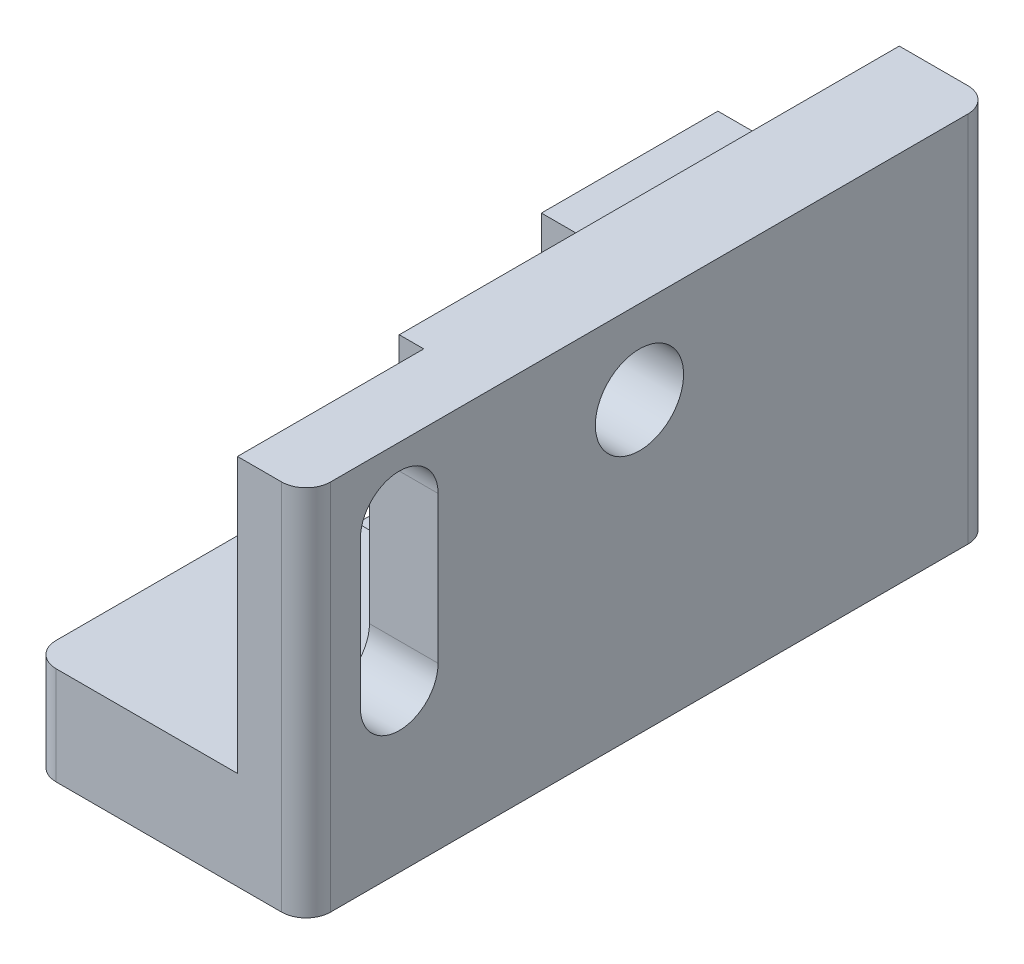
ISO-10303-21;
HEADER;
FILE_DESCRIPTION(('STEP AP214'),'2;1');
FILE_NAME('part.step','',(''),(''),'','','');
FILE_SCHEMA(('AUTOMOTIVE_DESIGN { 1 0 10303 214 1 1 1 1 }'));
ENDSEC;
DATA;
#1=APPLICATION_CONTEXT('core data for automotive mechanical design processes');
#2=APPLICATION_PROTOCOL_DEFINITION('international standard','automotive_design',2000,#1);
#3=PRODUCT_CONTEXT('',#1,'mechanical');
#4=PRODUCT('Part','Part','',(#3));
#5=PRODUCT_RELATED_PRODUCT_CATEGORY('part','',(#4));
#6=PRODUCT_DEFINITION_FORMATION('','',#4);
#7=PRODUCT_DEFINITION_CONTEXT('part definition',#1,'design');
#8=PRODUCT_DEFINITION('design','',#6,#7);
#9=PRODUCT_DEFINITION_SHAPE('','',#8);
#10=(LENGTH_UNIT() NAMED_UNIT(*) SI_UNIT(.MILLI.,.METRE.));
#11=(NAMED_UNIT(*) PLANE_ANGLE_UNIT() SI_UNIT($,.RADIAN.));
#12=(NAMED_UNIT(*) SI_UNIT($,.STERADIAN.) SOLID_ANGLE_UNIT());
#13=UNCERTAINTY_MEASURE_WITH_UNIT(LENGTH_MEASURE(1.E-05),#10,'distance_accuracy_value','');
#14=(GEOMETRIC_REPRESENTATION_CONTEXT(3) GLOBAL_UNCERTAINTY_ASSIGNED_CONTEXT((#13)) GLOBAL_UNIT_ASSIGNED_CONTEXT((#10,
#11,#12)) REPRESENTATION_CONTEXT('',''));
#15=CARTESIAN_POINT('',(0.,0.,0.));
#16=DIRECTION('',(0.,0.,1.));
#17=DIRECTION('',(1.,0.,0.));
#18=AXIS2_PLACEMENT_3D('',#15,#16,#17);
#19=CARTESIAN_POINT('',(-56.,20.,70.));
#20=DIRECTION('',(0.,-1.,0.));
#21=DIRECTION('',(0.,0.,-1.));
#22=AXIS2_PLACEMENT_3D('',#19,#20,#21);
#23=PLANE('',#22);
#24=DIRECTION('',(0.,0.,-1.));
#25=VECTOR('',#24,1.);
#26=CARTESIAN_POINT('',(-34.,20.,-16.4616556134456));
#27=LINE('',#26,#25);
#28=CARTESIAN_POINT('',(-34.,20.,13.5383443865544));
#29=VERTEX_POINT('',#28);
#30=CARTESIAN_POINT('',(-34.,20.,-16.4616556134456));
#31=VERTEX_POINT('',#30);
#32=EDGE_CURVE('E255',#29,#31,#27,.T.);
#33=ORIENTED_EDGE('',*,*,#32,.F.);
#34=DIRECTION('',(-1.,0.,0.));
#35=VECTOR('',#34,1.);
#36=CARTESIAN_POINT('',(-34.,20.,13.5383443865544));
#37=LINE('',#36,#35);
#38=CARTESIAN_POINT('',(-56.,20.,13.5383443865544));
#39=VERTEX_POINT('',#38);
#40=EDGE_CURVE('E269',#29,#39,#37,.T.);
#41=ORIENTED_EDGE('',*,*,#40,.T.);
#42=DIRECTION('',(0.,0.,-1.));
#43=VECTOR('',#42,1.);
#44=CARTESIAN_POINT('',(-56.,20.,70.));
#45=LINE('',#44,#43);
#46=CARTESIAN_POINT('',(-56.,20.,65.));
#47=VERTEX_POINT('',#46);
#48=EDGE_CURVE('E404',#47,#39,#45,.T.);
#49=ORIENTED_EDGE('',*,*,#48,.F.);
#50=CARTESIAN_POINT('',(-51.,20.,65.));
#51=DIRECTION('',(0.,-1.,0.));
#52=DIRECTION('',(0.,0.,1.));
#53=AXIS2_PLACEMENT_3D('',#50,#51,#52);
#54=CIRCLE('',#53,4.99999999999999);
#55=CARTESIAN_POINT('',(-51.,20.,70.));
#56=VERTEX_POINT('',#55);
#57=EDGE_CURVE('E352',#56,#47,#54,.T.);
#58=ORIENTED_EDGE('',*,*,#57,.F.);
#59=DIRECTION('',(-1.,0.,0.));
#60=VECTOR('',#59,1.);
#61=CARTESIAN_POINT('',(-56.,20.,70.));
#62=LINE('',#61,#60);
#63=CARTESIAN_POINT('',(-14.,20.,70.));
#64=VERTEX_POINT('',#63);
#65=EDGE_CURVE('E390',#64,#56,#62,.T.);
#66=ORIENTED_EDGE('',*,*,#65,.F.);
#67=DIRECTION('',(0.,0.,-1.));
#68=VECTOR('',#67,1.);
#69=CARTESIAN_POINT('',(-14.,20.,70.));
#70=LINE('',#69,#68);
#71=CARTESIAN_POINT('',(-14.,20.,32.));
#72=VERTEX_POINT('',#71);
#73=EDGE_CURVE('E410',#64,#72,#70,.T.);
#74=ORIENTED_EDGE('',*,*,#73,.T.);
#75=DIRECTION('',(1.,0.,0.));
#76=VECTOR('',#75,1.);
#77=CARTESIAN_POINT('',(-19.,20.,32.));
#78=LINE('',#77,#76);
#79=CARTESIAN_POINT('',(-19.,20.,32.));
#80=VERTEX_POINT('',#79);
#81=EDGE_CURVE('E351',#80,#72,#78,.T.);
#82=ORIENTED_EDGE('',*,*,#81,.F.);
#83=DIRECTION('',(0.,0.,1.));
#84=VECTOR('',#83,1.);
#85=CARTESIAN_POINT('',(-19.,20.,-70.));
#86=LINE('',#85,#84);
#87=CARTESIAN_POINT('',(-19.,20.,-34.));
#88=VERTEX_POINT('',#87);
#89=EDGE_CURVE('E339',#88,#80,#86,.T.);
#90=ORIENTED_EDGE('',*,*,#89,.F.);
#91=DIRECTION('',(-1.,0.,0.));
#92=VECTOR('',#91,1.);
#93=CARTESIAN_POINT('',(-19.,20.,-34.));
#94=LINE('',#93,#92);
#95=CARTESIAN_POINT('',(-56.,20.,-34.));
#96=VERTEX_POINT('',#95);
#97=EDGE_CURVE('E276',#88,#96,#94,.T.);
#98=ORIENTED_EDGE('',*,*,#97,.T.);
#99=CARTESIAN_POINT('',(-56.,20.,-16.4616556134456));
#100=VERTEX_POINT('',#99);
#101=EDGE_CURVE('E401',#100,#96,#45,.T.);
#102=ORIENTED_EDGE('',*,*,#101,.F.);
#103=DIRECTION('',(-1.,0.,0.));
#104=VECTOR('',#103,1.);
#105=CARTESIAN_POINT('',(-34.,20.,-16.4616556134456));
#106=LINE('',#105,#104);
#107=EDGE_CURVE('E65',#31,#100,#106,.T.);
#108=ORIENTED_EDGE('',*,*,#107,.F.);
#109=EDGE_LOOP('',(#33,#41,#49,#58,#66,#74,#82,#90,#98,#102,#108));
#110=FACE_BOUND('',#109,.T.);
#111=ADVANCED_FACE('F39',(#110),#23,.F.);
#112=CARTESIAN_POINT('',(-14.,20.,70.));
#113=DIRECTION('',(1.,0.,0.));
#114=DIRECTION('',(0.,0.,-1.));
#115=AXIS2_PLACEMENT_3D('',#112,#113,#114);
#116=PLANE('',#115);
#117=DIRECTION('',(0.,1.,0.));
#118=VECTOR('',#117,1.);
#119=CARTESIAN_POINT('',(-14.,33.,58.9234962612117));
#120=LINE('',#119,#118);
#121=CARTESIAN_POINT('',(-14.,33.,58.9234962612117));
#122=VERTEX_POINT('',#121);
#123=CARTESIAN_POINT('',(-14.,63.,58.9234962612117));
#124=VERTEX_POINT('',#123);
#125=EDGE_CURVE('E318',#122,#124,#120,.T.);
#126=ORIENTED_EDGE('',*,*,#125,.F.);
#127=CARTESIAN_POINT('',(-14.,33.,51.));
#128=DIRECTION('',(-1.,0.,0.));
#129=DIRECTION('',(0.,0.,1.));
#130=AXIS2_PLACEMENT_3D('',#127,#128,#129);
#131=CIRCLE('',#130,7.92349626121171);
#132=CARTESIAN_POINT('',(-14.,33.,43.0765037387883));
#133=VERTEX_POINT('',#132);
#134=EDGE_CURVE('E305',#133,#122,#131,.T.);
#135=ORIENTED_EDGE('',*,*,#134,.F.);
#136=DIRECTION('',(0.,-1.,0.));
#137=VECTOR('',#136,1.);
#138=CARTESIAN_POINT('',(-14.,33.,43.0765037387883));
#139=LINE('',#138,#137);
#140=CARTESIAN_POINT('',(-14.,63.,43.0765037387883));
#141=VERTEX_POINT('',#140);
#142=EDGE_CURVE('E307',#141,#133,#139,.T.);
#143=ORIENTED_EDGE('',*,*,#142,.F.);
#144=CARTESIAN_POINT('',(-14.,63.,51.));
#145=DIRECTION('',(-1.,0.,0.));
#146=DIRECTION('',(0.,0.,1.));
#147=AXIS2_PLACEMENT_3D('',#144,#145,#146);
#148=CIRCLE('',#147,7.92349626121171);
#149=EDGE_CURVE('E324',#124,#141,#148,.T.);
#150=ORIENTED_EDGE('',*,*,#149,.F.);
#151=EDGE_LOOP('',(#126,#135,#143,#150));
#152=FACE_BOUND('',#151,.T.);
#153=DIRECTION('',(0.,1.,0.));
#154=VECTOR('',#153,1.);
#155=CARTESIAN_POINT('',(-14.,76.,32.));
#156=LINE('',#155,#154);
#157=CARTESIAN_POINT('',(-14.,76.,32.));
#158=VERTEX_POINT('',#157);
#159=EDGE_CURVE('E326',#72,#158,#156,.T.);
#160=ORIENTED_EDGE('',*,*,#159,.F.);
#161=ORIENTED_EDGE('',*,*,#73,.F.);
#162=DIRECTION('',(0.,-1.,0.));
#163=VECTOR('',#162,1.);
#164=CARTESIAN_POINT('',(-14.,20.,70.));
#165=LINE('',#164,#163);
#166=CARTESIAN_POINT('',(-14.,76.,70.));
#167=VERTEX_POINT('',#166);
#168=EDGE_CURVE('E381',#167,#64,#165,.T.);
#169=ORIENTED_EDGE('',*,*,#168,.F.);
#170=DIRECTION('',(0.,0.,-1.));
#171=VECTOR('',#170,1.);
#172=CARTESIAN_POINT('',(-14.,76.,70.));
#173=LINE('',#172,#171);
#174=EDGE_CURVE('E408',#167,#158,#173,.T.);
#175=ORIENTED_EDGE('',*,*,#174,.T.);
#176=EDGE_LOOP('',(#160,#161,#169,#175));
#177=FACE_BOUND('',#176,.T.);
#178=ADVANCED_FACE('F450',(#152,#177),#116,.F.);
#179=CARTESIAN_POINT('',(-56.,0.,70.));
#180=DIRECTION('',(1.,0.,0.));
#181=DIRECTION('',(0.,0.,-1.));
#182=AXIS2_PLACEMENT_3D('',#179,#180,#181);
#183=PLANE('',#182);
#184=ORIENTED_EDGE('',*,*,#48,.T.);
#185=DIRECTION('',(0.,1.,0.));
#186=VECTOR('',#185,1.);
#187=CARTESIAN_POINT('',(-56.,9.99999999999999,13.5383443865544));
#188=LINE('',#187,#186);
#189=CARTESIAN_POINT('',(-56.,9.99999999999999,13.5383443865544));
#190=VERTEX_POINT('',#189);
#191=EDGE_CURVE('E257',#190,#39,#188,.T.);
#192=ORIENTED_EDGE('',*,*,#191,.F.);
#193=DIRECTION('',(0.,0.,1.));
#194=VECTOR('',#193,1.);
#195=CARTESIAN_POINT('',(-56.,9.99999999999999,-16.4616556134456));
#196=LINE('',#195,#194);
#197=CARTESIAN_POINT('',(-56.,9.99999999999999,-16.4616556134456));
#198=VERTEX_POINT('',#197);
#199=EDGE_CURVE('E266',#198,#190,#196,.T.);
#200=ORIENTED_EDGE('',*,*,#199,.F.);
#201=DIRECTION('',(0.,-1.,0.));
#202=VECTOR('',#201,1.);
#203=CARTESIAN_POINT('',(-56.,20.,-16.4616556134456));
#204=LINE('',#203,#202);
#205=EDGE_CURVE('E252',#100,#198,#204,.T.);
#206=ORIENTED_EDGE('',*,*,#205,.F.);
#207=ORIENTED_EDGE('',*,*,#101,.T.);
#208=DIRECTION('',(0.,1.,0.));
#209=VECTOR('',#208,1.);
#210=CARTESIAN_POINT('',(-56.,20.,-34.));
#211=LINE('',#210,#209);
#212=CARTESIAN_POINT('',(-56.,46.,-34.));
#213=VERTEX_POINT('',#212);
#214=EDGE_CURVE('E285',#96,#213,#211,.T.);
#215=ORIENTED_EDGE('',*,*,#214,.T.);
#216=DIRECTION('',(0.,0.,-1.));
#217=VECTOR('',#216,1.);
#218=CARTESIAN_POINT('',(-56.,46.,-34.));
#219=LINE('',#218,#217);
#220=CARTESIAN_POINT('',(-56.,46.,-70.));
#221=VERTEX_POINT('',#220);
#222=EDGE_CURVE('E289',#213,#221,#219,.T.);
#223=ORIENTED_EDGE('',*,*,#222,.T.);
#224=DIRECTION('',(0.,-1.,0.));
#225=VECTOR('',#224,1.);
#226=CARTESIAN_POINT('',(-56.,0.,-70.));
#227=LINE('',#226,#225);
#228=CARTESIAN_POINT('',(-56.,0.,-70.));
#229=VERTEX_POINT('',#228);
#230=EDGE_CURVE('E394',#221,#229,#227,.T.);
#231=ORIENTED_EDGE('',*,*,#230,.T.);
#232=DIRECTION('',(0.,0.,-1.));
#233=VECTOR('',#232,1.);
#234=CARTESIAN_POINT('',(-56.,0.,70.));
#235=LINE('',#234,#233);
#236=CARTESIAN_POINT('',(-56.,0.,65.));
#237=VERTEX_POINT('',#236);
#238=EDGE_CURVE('E402',#237,#229,#235,.T.);
#239=ORIENTED_EDGE('',*,*,#238,.F.);
#240=DIRECTION('',(0.,1.,0.));
#241=VECTOR('',#240,1.);
#242=CARTESIAN_POINT('',(-56.,-120.,65.));
#243=LINE('',#242,#241);
#244=EDGE_CURVE('E357',#237,#47,#243,.T.);
#245=ORIENTED_EDGE('',*,*,#244,.T.);
#246=EDGE_LOOP('',(#184,#192,#200,#206,#207,#215,#223,#231,#239,#245));
#247=FACE_BOUND('',#246,.T.);
#248=ADVANCED_FACE('F460',(#247),#183,.F.);
#249=CARTESIAN_POINT('',(0.,0.,70.));
#250=DIRECTION('',(0.,1.,0.));
#251=DIRECTION('',(-1.,0.,0.));
#252=AXIS2_PLACEMENT_3D('',#249,#250,#251);
#253=PLANE('',#252);
#254=CARTESIAN_POINT('',(-44.724100920092,0.,-1.46165561344556));
#255=DIRECTION('',(0.,1.,0.));
#256=DIRECTION('',(-1.,0.,0.));
#257=AXIS2_PLACEMENT_3D('',#254,#255,#256);
#258=CIRCLE('',#257,6.);
#259=CARTESIAN_POINT('',(-50.724100920092,0.,-1.46165561344556));
#260=VERTEX_POINT('',#259);
#261=EDGE_CURVE('E247',#260,#260,#258,.T.);
#262=ORIENTED_EDGE('',*,*,#261,.T.);
#263=EDGE_LOOP('',(#262));
#264=FACE_BOUND('',#263,.T.);
#265=DIRECTION('',(1.,0.,0.));
#266=VECTOR('',#265,1.);
#267=CARTESIAN_POINT('',(0.,0.,70.));
#268=LINE('',#267,#266);
#269=CARTESIAN_POINT('',(-51.,0.,70.));
#270=VERTEX_POINT('',#269);
#271=CARTESIAN_POINT('',(-5.,0.,70.));
#272=VERTEX_POINT('',#271);
#273=EDGE_CURVE('E388',#270,#272,#268,.T.);
#274=ORIENTED_EDGE('',*,*,#273,.F.);
#275=CARTESIAN_POINT('',(-51.,0.,65.));
#276=DIRECTION('',(0.,1.,0.));
#277=DIRECTION('',(-1.,0.,0.));
#278=AXIS2_PLACEMENT_3D('',#275,#276,#277);
#279=CIRCLE('',#278,4.99999999999999);
#280=EDGE_CURVE('E11',#270,#237,#279,.F.);
#281=ORIENTED_EDGE('',*,*,#280,.T.);
#282=ORIENTED_EDGE('',*,*,#238,.T.);
#283=DIRECTION('',(1.,0.,0.));
#284=VECTOR('',#283,1.);
#285=CARTESIAN_POINT('',(0.,0.,-70.));
#286=LINE('',#285,#284);
#287=CARTESIAN_POINT('',(-5.,0.,-70.));
#288=VERTEX_POINT('',#287);
#289=EDGE_CURVE('E383',#229,#288,#286,.T.);
#290=ORIENTED_EDGE('',*,*,#289,.T.);
#291=CARTESIAN_POINT('',(-5.,0.,-65.));
#292=DIRECTION('',(0.,-1.,0.));
#293=DIRECTION('',(0.,0.,1.));
#294=AXIS2_PLACEMENT_3D('',#291,#292,#293);
#295=CIRCLE('',#294,5.);
#296=CARTESIAN_POINT('',(0.,0.,-65.));
#297=VERTEX_POINT('',#296);
#298=EDGE_CURVE('E365',#288,#297,#295,.T.);
#299=ORIENTED_EDGE('',*,*,#298,.T.);
#300=DIRECTION('',(0.,0.,-1.));
#301=VECTOR('',#300,1.);
#302=CARTESIAN_POINT('',(0.,0.,70.));
#303=LINE('',#302,#301);
#304=CARTESIAN_POINT('',(0.,0.,65.));
#305=VERTEX_POINT('',#304);
#306=EDGE_CURVE('E395',#305,#297,#303,.T.);
#307=ORIENTED_EDGE('',*,*,#306,.F.);
#308=CARTESIAN_POINT('',(-5.,0.,65.));
#309=DIRECTION('',(0.,-1.,0.));
#310=DIRECTION('',(0.,0.,-1.));
#311=AXIS2_PLACEMENT_3D('',#308,#309,#310);
#312=CIRCLE('',#311,5.);
#313=EDGE_CURVE('E372',#305,#272,#312,.T.);
#314=ORIENTED_EDGE('',*,*,#313,.T.);
#315=EDGE_LOOP('',(#274,#281,#282,#290,#299,#307,#314));
#316=FACE_BOUND('',#315,.T.);
#317=ADVANCED_FACE('F430',(#264,#316),#253,.F.);
#318=CARTESIAN_POINT('',(0.,76.,70.));
#319=DIRECTION('',(-1.,0.,0.));
#320=DIRECTION('',(0.,0.,1.));
#321=AXIS2_PLACEMENT_3D('',#318,#319,#320);
#322=PLANE('',#321);
#323=CARTESIAN_POINT('',(0.,59.,2.00000000000001));
#324=DIRECTION('',(-1.,0.,0.));
#325=DIRECTION('',(0.,0.,1.));
#326=AXIS2_PLACEMENT_3D('',#323,#324,#325);
#327=CIRCLE('',#326,9.);
#328=CARTESIAN_POINT('',(0.,59.,11.));
#329=VERTEX_POINT('',#328);
#330=EDGE_CURVE('E299',#329,#329,#327,.T.);
#331=ORIENTED_EDGE('',*,*,#330,.T.);
#332=EDGE_LOOP('',(#331));
#333=FACE_BOUND('',#332,.T.);
#334=DIRECTION('',(0.,-1.,0.));
#335=VECTOR('',#334,1.);
#336=CARTESIAN_POINT('',(0.,33.,43.0765037387883));
#337=LINE('',#336,#335);
#338=CARTESIAN_POINT('',(0.,63.,43.0765037387883));
#339=VERTEX_POINT('',#338);
#340=CARTESIAN_POINT('',(0.,33.,43.0765037387883));
#341=VERTEX_POINT('',#340);
#342=EDGE_CURVE('E314',#339,#341,#337,.T.);
#343=ORIENTED_EDGE('',*,*,#342,.T.);
#344=CARTESIAN_POINT('',(0.,33.,51.));
#345=DIRECTION('',(-1.,0.,0.));
#346=DIRECTION('',(0.,0.,1.));
#347=AXIS2_PLACEMENT_3D('',#344,#345,#346);
#348=CIRCLE('',#347,7.92349626121171);
#349=CARTESIAN_POINT('',(0.,33.,58.9234962612117));
#350=VERTEX_POINT('',#349);
#351=EDGE_CURVE('E304',#341,#350,#348,.T.);
#352=ORIENTED_EDGE('',*,*,#351,.T.);
#353=DIRECTION('',(0.,1.,0.));
#354=VECTOR('',#353,1.);
#355=CARTESIAN_POINT('',(0.,33.,58.9234962612117));
#356=LINE('',#355,#354);
#357=CARTESIAN_POINT('',(0.,63.,58.9234962612117));
#358=VERTEX_POINT('',#357);
#359=EDGE_CURVE('E308',#350,#358,#356,.T.);
#360=ORIENTED_EDGE('',*,*,#359,.T.);
#361=CARTESIAN_POINT('',(0.,63.,51.));
#362=DIRECTION('',(-1.,0.,0.));
#363=DIRECTION('',(0.,0.,1.));
#364=AXIS2_PLACEMENT_3D('',#361,#362,#363);
#365=CIRCLE('',#364,7.92349626121171);
#366=EDGE_CURVE('E315',#358,#339,#365,.T.);
#367=ORIENTED_EDGE('',*,*,#366,.T.);
#368=EDGE_LOOP('',(#343,#352,#360,#367));
#369=FACE_BOUND('',#368,.T.);
#370=DIRECTION('',(0.,1.,0.));
#371=VECTOR('',#370,1.);
#372=CARTESIAN_POINT('',(0.,0.,-65.));
#373=LINE('',#372,#371);
#374=CARTESIAN_POINT('',(0.,76.,-65.));
#375=VERTEX_POINT('',#374);
#376=EDGE_CURVE('E367',#297,#375,#373,.T.);
#377=ORIENTED_EDGE('',*,*,#376,.T.);
#378=DIRECTION('',(0.,0.,-1.));
#379=VECTOR('',#378,1.);
#380=CARTESIAN_POINT('',(0.,76.,70.));
#381=LINE('',#380,#379);
#382=CARTESIAN_POINT('',(0.,76.,65.));
#383=VERTEX_POINT('',#382);
#384=EDGE_CURVE('E50',#383,#375,#381,.T.);
#385=ORIENTED_EDGE('',*,*,#384,.F.);
#386=DIRECTION('',(0.,1.,0.));
#387=VECTOR('',#386,1.);
#388=CARTESIAN_POINT('',(0.,0.,65.));
#389=LINE('',#388,#387);
#390=EDGE_CURVE('E380',#305,#383,#389,.T.);
#391=ORIENTED_EDGE('',*,*,#390,.F.);
#392=ORIENTED_EDGE('',*,*,#306,.T.);
#393=EDGE_LOOP('',(#377,#385,#391,#392));
#394=FACE_BOUND('',#393,.T.);
#395=ADVANCED_FACE('F41',(#333,#369,#394),#322,.F.);
#396=CARTESIAN_POINT('',(0.,0.,70.));
#397=DIRECTION('',(0.,0.,-1.));
#398=DIRECTION('',(-1.,0.,0.));
#399=AXIS2_PLACEMENT_3D('',#396,#397,#398);
#400=PLANE('',#399);
#401=ORIENTED_EDGE('',*,*,#65,.T.);
#402=DIRECTION('',(0.,1.,0.));
#403=VECTOR('',#402,1.);
#404=CARTESIAN_POINT('',(-51.,-120.,70.));
#405=LINE('',#404,#403);
#406=EDGE_CURVE('E358',#270,#56,#405,.T.);
#407=ORIENTED_EDGE('',*,*,#406,.F.);
#408=ORIENTED_EDGE('',*,*,#273,.T.);
#409=DIRECTION('',(0.,1.,0.));
#410=VECTOR('',#409,1.);
#411=CARTESIAN_POINT('',(-5.,0.,70.));
#412=LINE('',#411,#410);
#413=CARTESIAN_POINT('',(-5.,76.,70.));
#414=VERTEX_POINT('',#413);
#415=EDGE_CURVE('E368',#272,#414,#412,.T.);
#416=ORIENTED_EDGE('',*,*,#415,.T.);
#417=DIRECTION('',(-1.,0.,0.));
#418=VECTOR('',#417,1.);
#419=CARTESIAN_POINT('',(-14.,76.,70.));
#420=LINE('',#419,#418);
#421=EDGE_CURVE('E385',#414,#167,#420,.T.);
#422=ORIENTED_EDGE('',*,*,#421,.T.);
#423=ORIENTED_EDGE('',*,*,#168,.T.);
#424=EDGE_LOOP('',(#401,#407,#408,#416,#422,#423));
#425=FACE_BOUND('',#424,.T.);
#426=ADVANCED_FACE('F448',(#425),#400,.F.);
#427=CARTESIAN_POINT('',(0.,0.,-70.));
#428=DIRECTION('',(0.,0.,-1.));
#429=DIRECTION('',(-1.,0.,0.));
#430=AXIS2_PLACEMENT_3D('',#427,#428,#429);
#431=PLANE('',#430);
#432=ORIENTED_EDGE('',*,*,#230,.F.);
#433=DIRECTION('',(1.,0.,0.));
#434=VECTOR('',#433,1.);
#435=CARTESIAN_POINT('',(-56.,46.,-70.));
#436=LINE('',#435,#434);
#437=CARTESIAN_POINT('',(-19.,46.,-70.));
#438=VERTEX_POINT('',#437);
#439=EDGE_CURVE('E271',#221,#438,#436,.T.);
#440=ORIENTED_EDGE('',*,*,#439,.T.);
#441=DIRECTION('',(0.,-1.,0.));
#442=VECTOR('',#441,1.);
#443=CARTESIAN_POINT('',(-19.,76.,-70.));
#444=LINE('',#443,#442);
#445=CARTESIAN_POINT('',(-19.,76.,-70.));
#446=VERTEX_POINT('',#445);
#447=EDGE_CURVE('E340',#446,#438,#444,.T.);
#448=ORIENTED_EDGE('',*,*,#447,.F.);
#449=DIRECTION('',(-1.,0.,0.));
#450=VECTOR('',#449,1.);
#451=CARTESIAN_POINT('',(-14.,76.,-70.));
#452=LINE('',#451,#450);
#453=CARTESIAN_POINT('',(-5.,76.,-70.));
#454=VERTEX_POINT('',#453);
#455=EDGE_CURVE('E375',#454,#446,#452,.T.);
#456=ORIENTED_EDGE('',*,*,#455,.F.);
#457=DIRECTION('',(0.,1.,0.));
#458=VECTOR('',#457,1.);
#459=CARTESIAN_POINT('',(-5.,0.,-70.));
#460=LINE('',#459,#458);
#461=EDGE_CURVE('E362',#288,#454,#460,.T.);
#462=ORIENTED_EDGE('',*,*,#461,.F.);
#463=ORIENTED_EDGE('',*,*,#289,.F.);
#464=EDGE_LOOP('',(#432,#440,#448,#456,#462,#463));
#465=FACE_BOUND('',#464,.T.);
#466=ADVANCED_FACE('F431',(#465),#431,.T.);
#467=CARTESIAN_POINT('',(-14.,76.,70.));
#468=DIRECTION('',(0.,-1.,0.));
#469=DIRECTION('',(0.,0.,-1.));
#470=AXIS2_PLACEMENT_3D('',#467,#468,#469);
#471=PLANE('',#470);
#472=ORIENTED_EDGE('',*,*,#384,.T.);
#473=CARTESIAN_POINT('',(-5.,76.,-65.));
#474=DIRECTION('',(0.,-1.,0.));
#475=DIRECTION('',(0.,0.,1.));
#476=AXIS2_PLACEMENT_3D('',#473,#474,#475);
#477=CIRCLE('',#476,5.);
#478=EDGE_CURVE('E366',#454,#375,#477,.T.);
#479=ORIENTED_EDGE('',*,*,#478,.F.);
#480=ORIENTED_EDGE('',*,*,#455,.T.);
#481=DIRECTION('',(0.,0.,-1.));
#482=VECTOR('',#481,1.);
#483=CARTESIAN_POINT('',(-19.,76.,32.));
#484=LINE('',#483,#482);
#485=CARTESIAN_POINT('',(-19.,76.,32.));
#486=VERTEX_POINT('',#485);
#487=EDGE_CURVE('E344',#486,#446,#484,.T.);
#488=ORIENTED_EDGE('',*,*,#487,.F.);
#489=DIRECTION('',(1.,0.,0.));
#490=VECTOR('',#489,1.);
#491=CARTESIAN_POINT('',(-19.,76.,32.));
#492=LINE('',#491,#490);
#493=EDGE_CURVE('E347',#486,#158,#492,.T.);
#494=ORIENTED_EDGE('',*,*,#493,.T.);
#495=ORIENTED_EDGE('',*,*,#174,.F.);
#496=ORIENTED_EDGE('',*,*,#421,.F.);
#497=CARTESIAN_POINT('',(-5.,76.,65.));
#498=DIRECTION('',(0.,-1.,0.));
#499=DIRECTION('',(0.,0.,-1.));
#500=AXIS2_PLACEMENT_3D('',#497,#498,#499);
#501=CIRCLE('',#500,5.);
#502=EDGE_CURVE('E359',#383,#414,#501,.T.);
#503=ORIENTED_EDGE('',*,*,#502,.F.);
#504=EDGE_LOOP('',(#472,#479,#480,#488,#494,#495,#496,#503));
#505=FACE_BOUND('',#504,.T.);
#506=ADVANCED_FACE('F416',(#505),#471,.F.);
#507=CARTESIAN_POINT('',(-5.,0.,-65.));
#508=DIRECTION('',(0.,1.,0.));
#509=DIRECTION('',(0.,0.,1.));
#510=AXIS2_PLACEMENT_3D('',#507,#508,#509);
#511=CYLINDRICAL_SURFACE('',#510,5.);
#512=ORIENTED_EDGE('',*,*,#478,.T.);
#513=ORIENTED_EDGE('',*,*,#376,.F.);
#514=ORIENTED_EDGE('',*,*,#298,.F.);
#515=ORIENTED_EDGE('',*,*,#461,.T.);
#516=EDGE_LOOP('',(#512,#513,#514,#515));
#517=FACE_BOUND('',#516,.T.);
#518=ADVANCED_FACE('F421',(#517),#511,.T.);
#519=CARTESIAN_POINT('',(-5.,0.,65.));
#520=DIRECTION('',(0.,1.,0.));
#521=DIRECTION('',(0.,0.,1.));
#522=AXIS2_PLACEMENT_3D('',#519,#520,#521);
#523=CYLINDRICAL_SURFACE('',#522,5.);
#524=ORIENTED_EDGE('',*,*,#502,.T.);
#525=ORIENTED_EDGE('',*,*,#415,.F.);
#526=ORIENTED_EDGE('',*,*,#313,.F.);
#527=ORIENTED_EDGE('',*,*,#390,.T.);
#528=EDGE_LOOP('',(#524,#525,#526,#527));
#529=FACE_BOUND('',#528,.T.);
#530=ADVANCED_FACE('F451',(#529),#523,.T.);
#531=CARTESIAN_POINT('',(-51.,-120.,65.));
#532=DIRECTION('',(0.,1.,0.));
#533=DIRECTION('',(0.,0.,1.));
#534=AXIS2_PLACEMENT_3D('',#531,#532,#533);
#535=CYLINDRICAL_SURFACE('',#534,4.99999999999999);
#536=ORIENTED_EDGE('',*,*,#406,.T.);
#537=ORIENTED_EDGE('',*,*,#57,.T.);
#538=ORIENTED_EDGE('',*,*,#244,.F.);
#539=ORIENTED_EDGE('',*,*,#280,.F.);
#540=EDGE_LOOP('',(#536,#537,#538,#539));
#541=FACE_BOUND('',#540,.T.);
#542=ADVANCED_FACE('F546',(#541),#535,.T.);
#543=CARTESIAN_POINT('',(-19.,76.,32.));
#544=DIRECTION('',(0.,0.,-1.));
#545=DIRECTION('',(-1.,0.,0.));
#546=AXIS2_PLACEMENT_3D('',#543,#544,#545);
#547=PLANE('',#546);
#548=ORIENTED_EDGE('',*,*,#159,.T.);
#549=ORIENTED_EDGE('',*,*,#493,.F.);
#550=DIRECTION('',(0.,1.,0.));
#551=VECTOR('',#550,1.);
#552=CARTESIAN_POINT('',(-19.,76.,32.));
#553=LINE('',#552,#551);
#554=EDGE_CURVE('E342',#80,#486,#553,.T.);
#555=ORIENTED_EDGE('',*,*,#554,.F.);
#556=ORIENTED_EDGE('',*,*,#81,.T.);
#557=EDGE_LOOP('',(#548,#549,#555,#556));
#558=FACE_BOUND('',#557,.T.);
#559=ADVANCED_FACE('F445',(#558),#547,.F.);
#560=CARTESIAN_POINT('',(-19.,0.,0.));
#561=DIRECTION('',(-1.,0.,0.));
#562=DIRECTION('',(0.,0.,1.));
#563=AXIS2_PLACEMENT_3D('',#560,#561,#562);
#564=PLANE('',#563);
#565=DIRECTION('',(0.,0.,-1.));
#566=VECTOR('',#565,1.);
#567=CARTESIAN_POINT('',(-19.,46.,-34.));
#568=LINE('',#567,#566);
#569=CARTESIAN_POINT('',(-19.,46.,-34.));
#570=VERTEX_POINT('',#569);
#571=EDGE_CURVE('E291',#570,#438,#568,.T.);
#572=ORIENTED_EDGE('',*,*,#571,.F.);
#573=DIRECTION('',(0.,-1.,0.));
#574=VECTOR('',#573,1.);
#575=CARTESIAN_POINT('',(-19.,46.,-34.));
#576=LINE('',#575,#574);
#577=EDGE_CURVE('E288',#570,#88,#576,.T.);
#578=ORIENTED_EDGE('',*,*,#577,.T.);
#579=ORIENTED_EDGE('',*,*,#89,.T.);
#580=ORIENTED_EDGE('',*,*,#554,.T.);
#581=ORIENTED_EDGE('',*,*,#487,.T.);
#582=ORIENTED_EDGE('',*,*,#447,.T.);
#583=EDGE_LOOP('',(#572,#578,#579,#580,#581,#582));
#584=FACE_BOUND('',#583,.T.);
#585=CARTESIAN_POINT('',(-19.,59.,2.00000000000001));
#586=DIRECTION('',(-1.,0.,0.));
#587=DIRECTION('',(0.,0.,1.));
#588=AXIS2_PLACEMENT_3D('',#585,#586,#587);
#589=CIRCLE('',#588,9.);
#590=CARTESIAN_POINT('',(-19.,59.,11.));
#591=VERTEX_POINT('',#590);
#592=EDGE_CURVE('E298',#591,#591,#589,.T.);
#593=ORIENTED_EDGE('',*,*,#592,.F.);
#594=EDGE_LOOP('',(#593));
#595=FACE_BOUND('',#594,.T.);
#596=ADVANCED_FACE('F434',(#584,#595),#564,.T.);
#597=CARTESIAN_POINT('',(0.,33.,51.));
#598=DIRECTION('',(-1.,0.,0.));
#599=DIRECTION('',(0.,0.,1.));
#600=AXIS2_PLACEMENT_3D('',#597,#598,#599);
#601=CYLINDRICAL_SURFACE('',#600,7.92349626121171);
#602=ORIENTED_EDGE('',*,*,#134,.T.);
#603=DIRECTION('',(-1.,0.,0.));
#604=VECTOR('',#603,1.);
#605=CARTESIAN_POINT('',(0.,33.,58.9234962612117));
#606=LINE('',#605,#604);
#607=EDGE_CURVE('E319',#350,#122,#606,.T.);
#608=ORIENTED_EDGE('',*,*,#607,.F.);
#609=ORIENTED_EDGE('',*,*,#351,.F.);
#610=DIRECTION('',(-1.,0.,0.));
#611=VECTOR('',#610,1.);
#612=CARTESIAN_POINT('',(0.,33.,43.0765037387883));
#613=LINE('',#612,#611);
#614=EDGE_CURVE('E328',#341,#133,#613,.T.);
#615=ORIENTED_EDGE('',*,*,#614,.T.);
#616=EDGE_LOOP('',(#602,#608,#609,#615));
#617=FACE_BOUND('',#616,.T.);
#618=ADVANCED_FACE('F555',(#617),#601,.F.);
#619=CARTESIAN_POINT('',(0.,33.,43.0765037387883));
#620=DIRECTION('',(0.,0.,-1.));
#621=DIRECTION('',(0.,1.,0.));
#622=AXIS2_PLACEMENT_3D('',#619,#620,#621);
#623=PLANE('',#622);
#624=ORIENTED_EDGE('',*,*,#142,.T.);
#625=ORIENTED_EDGE('',*,*,#614,.F.);
#626=ORIENTED_EDGE('',*,*,#342,.F.);
#627=DIRECTION('',(-1.,0.,0.));
#628=VECTOR('',#627,1.);
#629=CARTESIAN_POINT('',(0.,63.,43.0765037387883));
#630=LINE('',#629,#628);
#631=EDGE_CURVE('E331',#339,#141,#630,.T.);
#632=ORIENTED_EDGE('',*,*,#631,.T.);
#633=EDGE_LOOP('',(#624,#625,#626,#632));
#634=FACE_BOUND('',#633,.T.);
#635=ADVANCED_FACE('F560',(#634),#623,.F.);
#636=CARTESIAN_POINT('',(0.,63.,51.));
#637=DIRECTION('',(-1.,0.,0.));
#638=DIRECTION('',(0.,0.,1.));
#639=AXIS2_PLACEMENT_3D('',#636,#637,#638);
#640=CYLINDRICAL_SURFACE('',#639,7.92349626121171);
#641=ORIENTED_EDGE('',*,*,#149,.T.);
#642=ORIENTED_EDGE('',*,*,#631,.F.);
#643=ORIENTED_EDGE('',*,*,#366,.F.);
#644=DIRECTION('',(-1.,0.,0.));
#645=VECTOR('',#644,1.);
#646=CARTESIAN_POINT('',(0.,63.,58.9234962612117));
#647=LINE('',#646,#645);
#648=EDGE_CURVE('E333',#358,#124,#647,.T.);
#649=ORIENTED_EDGE('',*,*,#648,.T.);
#650=EDGE_LOOP('',(#641,#642,#643,#649));
#651=FACE_BOUND('',#650,.T.);
#652=ADVANCED_FACE('F565',(#651),#640,.F.);
#653=CARTESIAN_POINT('',(0.,33.,58.9234962612117));
#654=DIRECTION('',(0.,0.,1.));
#655=DIRECTION('',(0.,-1.,0.));
#656=AXIS2_PLACEMENT_3D('',#653,#654,#655);
#657=PLANE('',#656);
#658=ORIENTED_EDGE('',*,*,#125,.T.);
#659=ORIENTED_EDGE('',*,*,#648,.F.);
#660=ORIENTED_EDGE('',*,*,#359,.F.);
#661=ORIENTED_EDGE('',*,*,#607,.T.);
#662=EDGE_LOOP('',(#658,#659,#660,#661));
#663=FACE_BOUND('',#662,.T.);
#664=ADVANCED_FACE('F559',(#663),#657,.F.);
#665=CARTESIAN_POINT('',(0.,59.,2.00000000000001));
#666=DIRECTION('',(-1.,0.,0.));
#667=DIRECTION('',(0.,0.,1.));
#668=AXIS2_PLACEMENT_3D('',#665,#666,#667);
#669=CYLINDRICAL_SURFACE('',#668,9.);
#670=ORIENTED_EDGE('',*,*,#330,.F.);
#671=EDGE_LOOP('',(#670));
#672=FACE_BOUND('',#671,.T.);
#673=ORIENTED_EDGE('',*,*,#592,.T.);
#674=EDGE_LOOP('',(#673));
#675=FACE_BOUND('',#674,.T.);
#676=ADVANCED_FACE('F482',(#672,#675),#669,.F.);
#677=CARTESIAN_POINT('',(-56.,46.,-34.));
#678=DIRECTION('',(0.,1.,0.));
#679=DIRECTION('',(-1.,0.,0.));
#680=AXIS2_PLACEMENT_3D('',#677,#678,#679);
#681=PLANE('',#680);
#682=ORIENTED_EDGE('',*,*,#439,.F.);
#683=ORIENTED_EDGE('',*,*,#222,.F.);
#684=DIRECTION('',(1.,0.,0.));
#685=VECTOR('',#684,1.);
#686=CARTESIAN_POINT('',(-56.,46.,-34.));
#687=LINE('',#686,#685);
#688=EDGE_CURVE('E281',#213,#570,#687,.T.);
#689=ORIENTED_EDGE('',*,*,#688,.T.);
#690=ORIENTED_EDGE('',*,*,#571,.T.);
#691=EDGE_LOOP('',(#682,#683,#689,#690));
#692=FACE_BOUND('',#691,.T.);
#693=ADVANCED_FACE('F463',(#692),#681,.T.);
#694=CARTESIAN_POINT('',(0.,0.,-34.));
#695=DIRECTION('',(0.,0.,-1.));
#696=DIRECTION('',(-1.,0.,0.));
#697=AXIS2_PLACEMENT_3D('',#694,#695,#696);
#698=PLANE('',#697);
#699=DIRECTION('',(1.,0.,0.));
#700=VECTOR('',#699,1.);
#701=CARTESIAN_POINT('',(-45.5,27.6782717280586,-34.));
#702=LINE('',#701,#700);
#703=CARTESIAN_POINT('',(-45.5,27.6782717280586,-34.));
#704=VERTEX_POINT('',#703);
#705=CARTESIAN_POINT('',(-28.5,27.6782717280586,-34.));
#706=VERTEX_POINT('',#705);
#707=EDGE_CURVE('E236',#704,#706,#702,.T.);
#708=ORIENTED_EDGE('',*,*,#707,.F.);
#709=CARTESIAN_POINT('',(-45.5,33.6782717280586,-34.));
#710=DIRECTION('',(0.,0.,1.));
#711=DIRECTION('',(1.,0.,0.));
#712=AXIS2_PLACEMENT_3D('',#709,#710,#711);
#713=CIRCLE('',#712,6.);
#714=CARTESIAN_POINT('',(-45.5,39.6782717280586,-34.));
#715=VERTEX_POINT('',#714);
#716=EDGE_CURVE('E53',#715,#704,#713,.T.);
#717=ORIENTED_EDGE('',*,*,#716,.F.);
#718=DIRECTION('',(-1.,0.,0.));
#719=VECTOR('',#718,1.);
#720=CARTESIAN_POINT('',(-45.5,39.6782717280586,-34.));
#721=LINE('',#720,#719);
#722=CARTESIAN_POINT('',(-28.5,39.6782717280586,-34.));
#723=VERTEX_POINT('',#722);
#724=EDGE_CURVE('E227',#723,#715,#721,.T.);
#725=ORIENTED_EDGE('',*,*,#724,.F.);
#726=CARTESIAN_POINT('',(-28.5,33.6782717280586,-34.));
#727=DIRECTION('',(0.,0.,1.));
#728=DIRECTION('',(1.,0.,0.));
#729=AXIS2_PLACEMENT_3D('',#726,#727,#728);
#730=CIRCLE('',#729,6.);
#731=EDGE_CURVE('E229',#706,#723,#730,.T.);
#732=ORIENTED_EDGE('',*,*,#731,.F.);
#733=EDGE_LOOP('',(#708,#717,#725,#732));
#734=FACE_BOUND('',#733,.T.);
#735=ORIENTED_EDGE('',*,*,#97,.F.);
#736=ORIENTED_EDGE('',*,*,#577,.F.);
#737=ORIENTED_EDGE('',*,*,#688,.F.);
#738=ORIENTED_EDGE('',*,*,#214,.F.);
#739=EDGE_LOOP('',(#735,#736,#737,#738));
#740=FACE_BOUND('',#739,.T.);
#741=ADVANCED_FACE('F468',(#734,#740),#698,.F.);
#742=CARTESIAN_POINT('',(-34.,9.99999999999999,13.5383443865544));
#743=DIRECTION('',(0.,0.,1.));
#744=DIRECTION('',(1.,0.,0.));
#745=AXIS2_PLACEMENT_3D('',#742,#743,#744);
#746=PLANE('',#745);
#747=ORIENTED_EDGE('',*,*,#191,.T.);
#748=ORIENTED_EDGE('',*,*,#40,.F.);
#749=DIRECTION('',(0.,1.,0.));
#750=VECTOR('',#749,1.);
#751=CARTESIAN_POINT('',(-34.,9.99999999999999,13.5383443865544));
#752=LINE('',#751,#750);
#753=CARTESIAN_POINT('',(-34.,9.99999999999999,13.5383443865544));
#754=VERTEX_POINT('',#753);
#755=EDGE_CURVE('E265',#754,#29,#752,.T.);
#756=ORIENTED_EDGE('',*,*,#755,.F.);
#757=DIRECTION('',(-1.,0.,0.));
#758=VECTOR('',#757,1.);
#759=CARTESIAN_POINT('',(-34.,9.99999999999999,13.5383443865544));
#760=LINE('',#759,#758);
#761=EDGE_CURVE('E274',#754,#190,#760,.T.);
#762=ORIENTED_EDGE('',*,*,#761,.T.);
#763=EDGE_LOOP('',(#747,#748,#756,#762));
#764=FACE_BOUND('',#763,.T.);
#765=ADVANCED_FACE('F475',(#764),#746,.F.);
#766=CARTESIAN_POINT('',(-34.,9.99999999999999,-16.4616556134456));
#767=DIRECTION('',(0.,-1.,0.));
#768=DIRECTION('',(0.,0.,-1.));
#769=AXIS2_PLACEMENT_3D('',#766,#767,#768);
#770=PLANE('',#769);
#771=CARTESIAN_POINT('',(-44.724100920092,9.99999999999999,-1.46165561344556));
#772=DIRECTION('',(0.,1.,0.));
#773=DIRECTION('',(0.,0.,1.));
#774=AXIS2_PLACEMENT_3D('',#771,#772,#773);
#775=CIRCLE('',#774,6.);
#776=CARTESIAN_POINT('',(-44.724100920092,9.99999999999999,4.53834438655444));
#777=VERTEX_POINT('',#776);
#778=EDGE_CURVE('E245',#777,#777,#775,.T.);
#779=ORIENTED_EDGE('',*,*,#778,.F.);
#780=EDGE_LOOP('',(#779));
#781=FACE_BOUND('',#780,.T.);
#782=ORIENTED_EDGE('',*,*,#199,.T.);
#783=ORIENTED_EDGE('',*,*,#761,.F.);
#784=DIRECTION('',(0.,0.,1.));
#785=VECTOR('',#784,1.);
#786=CARTESIAN_POINT('',(-34.,9.99999999999999,-16.4616556134456));
#787=LINE('',#786,#785);
#788=CARTESIAN_POINT('',(-34.,9.99999999999999,-16.4616556134456));
#789=VERTEX_POINT('',#788);
#790=EDGE_CURVE('E256',#789,#754,#787,.T.);
#791=ORIENTED_EDGE('',*,*,#790,.F.);
#792=DIRECTION('',(-1.,0.,0.));
#793=VECTOR('',#792,1.);
#794=CARTESIAN_POINT('',(-34.,9.99999999999999,-16.4616556134456));
#795=LINE('',#794,#793);
#796=EDGE_CURVE('E277',#789,#198,#795,.T.);
#797=ORIENTED_EDGE('',*,*,#796,.T.);
#798=EDGE_LOOP('',(#782,#783,#791,#797));
#799=FACE_BOUND('',#798,.T.);
#800=ADVANCED_FACE('F476',(#781,#799),#770,.F.);
#801=CARTESIAN_POINT('',(-34.,20.,-16.4616556134456));
#802=DIRECTION('',(0.,0.,-1.));
#803=DIRECTION('',(-1.,0.,0.));
#804=AXIS2_PLACEMENT_3D('',#801,#802,#803);
#805=PLANE('',#804);
#806=ORIENTED_EDGE('',*,*,#205,.T.);
#807=ORIENTED_EDGE('',*,*,#796,.F.);
#808=DIRECTION('',(0.,-1.,0.));
#809=VECTOR('',#808,1.);
#810=CARTESIAN_POINT('',(-34.,20.,-16.4616556134456));
#811=LINE('',#810,#809);
#812=EDGE_CURVE('E253',#31,#789,#811,.T.);
#813=ORIENTED_EDGE('',*,*,#812,.F.);
#814=ORIENTED_EDGE('',*,*,#107,.T.);
#815=EDGE_LOOP('',(#806,#807,#813,#814));
#816=FACE_BOUND('',#815,.T.);
#817=ADVANCED_FACE('F532',(#816),#805,.F.);
#818=CARTESIAN_POINT('',(-34.,0.,0.));
#819=DIRECTION('',(-1.,0.,0.));
#820=DIRECTION('',(0.,0.,1.));
#821=AXIS2_PLACEMENT_3D('',#818,#819,#820);
#822=PLANE('',#821);
#823=ORIENTED_EDGE('',*,*,#32,.T.);
#824=ORIENTED_EDGE('',*,*,#812,.T.);
#825=ORIENTED_EDGE('',*,*,#790,.T.);
#826=ORIENTED_EDGE('',*,*,#755,.T.);
#827=EDGE_LOOP('',(#823,#824,#825,#826));
#828=FACE_BOUND('',#827,.T.);
#829=ADVANCED_FACE('F524',(#828),#822,.T.);
#830=CARTESIAN_POINT('',(-44.724100920092,-12.,-1.46165561344556));
#831=DIRECTION('',(0.,1.,0.));
#832=DIRECTION('',(0.,0.,1.));
#833=AXIS2_PLACEMENT_3D('',#830,#831,#832);
#834=CYLINDRICAL_SURFACE('',#833,6.);
#835=ORIENTED_EDGE('',*,*,#778,.T.);
#836=EDGE_LOOP('',(#835));
#837=FACE_BOUND('',#836,.T.);
#838=ORIENTED_EDGE('',*,*,#261,.F.);
#839=EDGE_LOOP('',(#838));
#840=FACE_BOUND('',#839,.T.);
#841=ADVANCED_FACE('F523',(#837,#840),#834,.F.);
#842=CARTESIAN_POINT('',(-45.5,33.6782717280586,-56.));
#843=DIRECTION('',(0.,0.,1.));
#844=DIRECTION('',(1.,0.,0.));
#845=AXIS2_PLACEMENT_3D('',#842,#843,#844);
#846=CYLINDRICAL_SURFACE('',#845,6.);
#847=ORIENTED_EDGE('',*,*,#716,.T.);
#848=DIRECTION('',(0.,0.,1.));
#849=VECTOR('',#848,1.);
#850=CARTESIAN_POINT('',(-45.5,27.6782717280586,-56.));
#851=LINE('',#850,#849);
#852=CARTESIAN_POINT('',(-45.5,27.6782717280586,-56.));
#853=VERTEX_POINT('',#852);
#854=EDGE_CURVE('E204',#853,#704,#851,.T.);
#855=ORIENTED_EDGE('',*,*,#854,.F.);
#856=CARTESIAN_POINT('',(-45.5,33.6782717280586,-56.));
#857=DIRECTION('',(0.,0.,1.));
#858=DIRECTION('',(1.,0.,0.));
#859=AXIS2_PLACEMENT_3D('',#856,#857,#858);
#860=CIRCLE('',#859,6.);
#861=CARTESIAN_POINT('',(-45.5,39.6782717280586,-56.));
#862=VERTEX_POINT('',#861);
#863=EDGE_CURVE('E209',#862,#853,#860,.T.);
#864=ORIENTED_EDGE('',*,*,#863,.F.);
#865=DIRECTION('',(0.,0.,1.));
#866=VECTOR('',#865,1.);
#867=CARTESIAN_POINT('',(-45.5,39.6782717280586,-56.));
#868=LINE('',#867,#866);
#869=EDGE_CURVE('E239',#862,#715,#868,.T.);
#870=ORIENTED_EDGE('',*,*,#869,.T.);
#871=EDGE_LOOP('',(#847,#855,#864,#870));
#872=FACE_BOUND('',#871,.T.);
#873=ADVANCED_FACE('F210',(#872),#846,.F.);
#874=CARTESIAN_POINT('',(-45.5,39.6782717280586,-56.));
#875=DIRECTION('',(0.,1.,0.));
#876=DIRECTION('',(0.,0.,1.));
#877=AXIS2_PLACEMENT_3D('',#874,#875,#876);
#878=PLANE('',#877);
#879=ORIENTED_EDGE('',*,*,#724,.T.);
#880=ORIENTED_EDGE('',*,*,#869,.F.);
#881=DIRECTION('',(-1.,0.,0.));
#882=VECTOR('',#881,1.);
#883=CARTESIAN_POINT('',(-45.5,39.6782717280586,-56.));
#884=LINE('',#883,#882);
#885=CARTESIAN_POINT('',(-28.5,39.6782717280586,-56.));
#886=VERTEX_POINT('',#885);
#887=EDGE_CURVE('E213',#886,#862,#884,.T.);
#888=ORIENTED_EDGE('',*,*,#887,.F.);
#889=DIRECTION('',(0.,0.,1.));
#890=VECTOR('',#889,1.);
#891=CARTESIAN_POINT('',(-28.5,39.6782717280586,-56.));
#892=LINE('',#891,#890);
#893=EDGE_CURVE('E243',#886,#723,#892,.T.);
#894=ORIENTED_EDGE('',*,*,#893,.T.);
#895=EDGE_LOOP('',(#879,#880,#888,#894));
#896=FACE_BOUND('',#895,.T.);
#897=ADVANCED_FACE('F527',(#896),#878,.F.);
#898=CARTESIAN_POINT('',(-28.5,33.6782717280586,-56.));
#899=DIRECTION('',(0.,0.,1.));
#900=DIRECTION('',(1.,0.,0.));
#901=AXIS2_PLACEMENT_3D('',#898,#899,#900);
#902=CYLINDRICAL_SURFACE('',#901,6.);
#903=ORIENTED_EDGE('',*,*,#731,.T.);
#904=ORIENTED_EDGE('',*,*,#893,.F.);
#905=CARTESIAN_POINT('',(-28.5,33.6782717280586,-56.));
#906=DIRECTION('',(0.,0.,1.));
#907=DIRECTION('',(1.,0.,0.));
#908=AXIS2_PLACEMENT_3D('',#905,#906,#907);
#909=CIRCLE('',#908,6.);
#910=CARTESIAN_POINT('',(-28.5,27.6782717280586,-56.));
#911=VERTEX_POINT('',#910);
#912=EDGE_CURVE('E223',#911,#886,#909,.T.);
#913=ORIENTED_EDGE('',*,*,#912,.F.);
#914=DIRECTION('',(0.,0.,1.));
#915=VECTOR('',#914,1.);
#916=CARTESIAN_POINT('',(-28.5,27.6782717280586,-56.));
#917=LINE('',#916,#915);
#918=EDGE_CURVE('E211',#911,#706,#917,.T.);
#919=ORIENTED_EDGE('',*,*,#918,.T.);
#920=EDGE_LOOP('',(#903,#904,#913,#919));
#921=FACE_BOUND('',#920,.T.);
#922=ADVANCED_FACE('F690',(#921),#902,.F.);
#923=CARTESIAN_POINT('',(-45.5,27.6782717280586,-56.));
#924=DIRECTION('',(0.,-1.,0.));
#925=DIRECTION('',(0.,0.,-1.));
#926=AXIS2_PLACEMENT_3D('',#923,#924,#925);
#927=PLANE('',#926);
#928=ORIENTED_EDGE('',*,*,#707,.T.);
#929=ORIENTED_EDGE('',*,*,#918,.F.);
#930=DIRECTION('',(1.,0.,0.));
#931=VECTOR('',#930,1.);
#932=CARTESIAN_POINT('',(-45.5,27.6782717280586,-56.));
#933=LINE('',#932,#931);
#934=EDGE_CURVE('E218',#853,#911,#933,.T.);
#935=ORIENTED_EDGE('',*,*,#934,.F.);
#936=ORIENTED_EDGE('',*,*,#854,.T.);
#937=EDGE_LOOP('',(#928,#929,#935,#936));
#938=FACE_BOUND('',#937,.T.);
#939=ADVANCED_FACE('F219',(#938),#927,.F.);
#940=CARTESIAN_POINT('',(-45.5,33.6782717280586,-56.));
#941=DIRECTION('',(0.,0.,1.));
#942=DIRECTION('',(1.,0.,0.));
#943=AXIS2_PLACEMENT_3D('',#940,#941,#942);
#944=PLANE('',#943);
#945=ORIENTED_EDGE('',*,*,#863,.T.);
#946=ORIENTED_EDGE('',*,*,#934,.T.);
#947=ORIENTED_EDGE('',*,*,#912,.T.);
#948=ORIENTED_EDGE('',*,*,#887,.T.);
#949=EDGE_LOOP('',(#945,#946,#947,#948));
#950=FACE_BOUND('',#949,.T.);
#951=ADVANCED_FACE('F224',(#950),#944,.T.);
#952=CLOSED_SHELL('',(#111,#178,#248,#317,#395,#426,#466,#506,#518,#530,#542,#559,#596,#618,
#635,#652,#664,#676,#693,#741,#765,#800,#817,#829,#841,#873,#897,#922,#939,#951));
#953=MANIFOLD_SOLID_BREP('B2',#952);
#954=ADVANCED_BREP_SHAPE_REPRESENTATION('',(#18,#953),#14);
#955=SHAPE_DEFINITION_REPRESENTATION(#9,#954);
ENDSEC;
END-ISO-10303-21;
